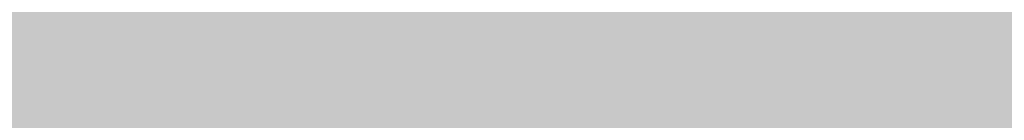
# Model space of a CAD drawing. Units: feet. Extents: x 3168 to 4724, y 827 to 1477.
# Tile 217 of 256: x 3363.87 to 3379.08, y 1096.78 to 1098.34. Entities that reach past the tile are written whole.
import ezdxf

# ---------------------------------------------------------------- set-up
doc = ezdxf.new("R2010")
doc.units = ezdxf.units.FT
doc.layers.add('A-ELEV-PATT', color=8, linetype='Continuous', lineweight=13)

msp = doc.modelspace()

# ---------------------------------------------------------------- hatches: boundary and pattern name
at = {"layer": 'A-ELEV-PATT'}
h = msp.add_hatch(color=256, dxfattribs=at)
h.dxf.hatch_style = 1
edge = h.paths.add_edge_path()
edge.add_ellipse((3552.906, 979.22), major_axis=(36.745, 0), ratio=0.484848, start_angle=0, end_angle=360)
edge = h.paths.add_edge_path()
edge.add_ellipse((3559.892, 929.252), major_axis=(36.745, 0), ratio=0.484848, start_angle=0, end_angle=360)
edge = h.paths.add_edge_path()
edge.add_line((3299.317, 1198.606), (3479.917, 1198.606))
edge.add_line((3479.917, 1198.606), (3479.917, 1209.869))
edge.add_spline(control_points=[(3479.917, 1209.869), (3464.301, 1209.869), (3448.686, 1209.869), (3410.949, 1209.869), (3388.828, 1209.869), (3355.647, 1209.869), (3344.586, 1209.869), (3327.996, 1209.869), (3322.466, 1209.869), (3314.17, 1209.869), (3311.405, 1209.869), (3307.257, 1209.869), (3305.875, 1209.869), (3303.801, 1209.869), (3303.11, 1209.869), (3302.073, 1209.869), (3301.727, 1209.869), (3301.209, 1209.869), (3301.036, 1209.869), (3300.777, 1209.869), (3300.69, 1209.869), (3300.561, 1209.869), (3300.517, 1209.869), (3300.453, 1209.869), (3300.431, 1209.869), (3300.399, 1209.869), (3300.388, 1209.869), (3300.366, 1209.869), (3300.346, 1209.869), (3300.346, 1209.869), (3300.346, 1209.869), (3300.343, 1209.869), (3300.341, 1209.869), (3300.338, 1209.869), (3300.337, 1209.869), (3300.334, 1209.869), (3300.332, 1209.869), (3300.326, 1209.869), (3300.321, 1209.869), (3300.311, 1209.869), (3300.306, 1209.869), (3300.291, 1209.869), (3300.28, 1209.869), (3300.232, 1209.869), (3300.195, 1209.869), (3299.951, 1209.871), (3299.745, 1209.874), (3299.437, 1209.883), (3299.334, 1209.887), (3299.181, 1209.893), (3299.13, 1209.895), (3298.652, 1209.917), (3298.229, 1209.946), (3297.602, 1210.002), (3297.393, 1210.023), (3297.083, 1210.058), (3296.979, 1210.07), (3296.293, 1210.155), (3295.718, 1210.243), (3294.869, 1210.399), (3294.588, 1210.454), (3294.169, 1210.543), (3294.03, 1210.574), (3291.707, 1211.101), (3289.654, 1211.813), (3285.776, 1213.564), (3283.951, 1214.603), (3280.512, 1216.98), (3278.897, 1218.318), (3276.38, 1220.829), (3275.416, 1221.918), (3274.039, 1223.708), (3273.581, 1224.35), (3273.143, 1225.016)], knot_values=[39.119033, 39.119033, 39.119033, 39.119033, 39.286353, 39.286353, 39.523379, 39.523379, 39.641892, 39.641892, 39.701148, 39.701148, 39.730777, 39.730777, 39.745591, 39.745591, 39.752998, 39.752998, 39.756701, 39.756701, 39.758553, 39.758553, 39.759479, 39.759479, 39.759942, 39.759942, 39.760173, 39.760173, 39.760289, 39.760289, 39.760405, 39.760405, 39.760463, 39.760463, 39.763389, 39.763389, 39.764851, 39.764851, 39.767304, 39.767304, 39.773825, 39.773825, 39.78057, 39.78057, 39.79477, 39.79477, 39.845194, 39.845194, 40.126715, 40.126715, 40.267476, 40.267476, 40.337856, 40.337856, 40.927023, 40.927023, 41.221606, 41.221606, 41.368898, 41.368898, 42.202622, 42.202622, 42.619485, 42.619485, 42.827916, 42.827916, 46.118323, 46.118323, 49.408731, 49.408731, 52.699139, 52.699139, 54.927489, 54.927489, 56.104228, 56.104228, 56.104228, 56.104228], weights=[1, 1, 1, 1, 1, 1, 1, 1, 1, 1, 1, 1, 1, 1, 1, 1, 1, 1, 1, 1, 1, 1, 1, 1, 1, 1, 1, 1, 1, 1, 1, 1, 1, 1, 1, 1, 1, 1, 1, 1, 1, 1, 1, 1, 1, 1, 1, 1, 1, 1, 1, 1, 1, 1, 1, 1, 1, 1, 1, 1, 1, 1, 1, 1, 1, 1, 1, 1, 1, 1, 1, 1, 1, 1], degree=3, periodic=0)
edge.add_line((3273.143, 1225.016), (3273.143, 1099.016))
edge.add_line((3273.143, 1099.016), (3299.317, 1099.016))
edge.add_line((3299.317, 1099.016), (3299.317, 1198.606))
edge = h.paths.add_edge_path()
edge.add_line((3304.758, 1324.158), (3479.917, 1324.158))
edge.add_line((3479.917, 1324.158), (3479.917, 1335.715))
edge.add_line((3479.917, 1335.715), (3269.162, 1335.715))
edge.add_spline(control_points=[(3269.162, 1335.715), (3264.024, 1335.715), (3258.364, 1328.958), (3259.264, 1323.9)], knot_values=[0, 0, 0, 0, 15.412191, 15.412191, 15.412191, 15.412191], degree=3, periodic=0)
edge.add_line((3259.264, 1323.9), (3265.517, 1288.769))
edge.add_line((3265.517, 1288.769), (3275.265, 1261.546))
edge.add_line((3275.265, 1261.546), (3304.758, 1261.546))
edge.add_line((3304.758, 1261.546), (3304.758, 1324.158))
h = msp.add_hatch(color=256, dxfattribs=at)
h.dxf.hatch_style = 1
h.paths.add_polyline_path([(3384.525, 1099.016), (3335.029, 1099.016), (3299.317, 1099.016), (3273.143, 1099.016), (3217.565, 1099.016), (3168.069, 827.116), (3335.029, 827.116)])

doc.saveas('drawing.dxf')
